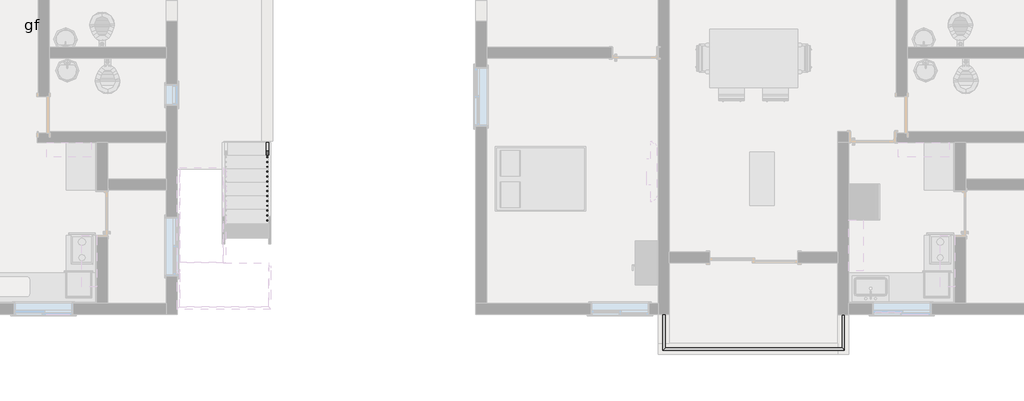
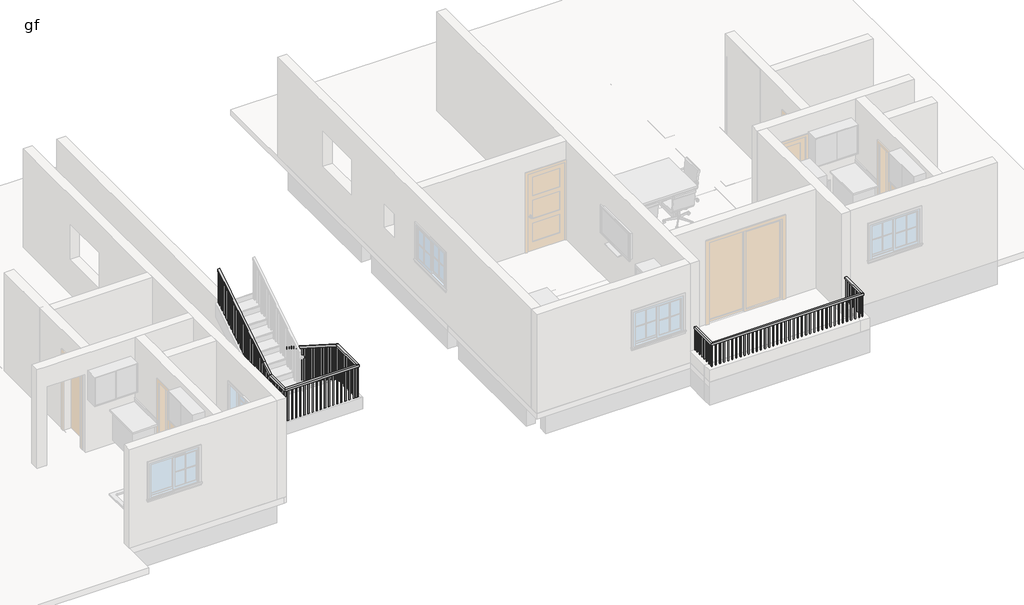
# One storey, part 5 of 8: 2 railings.
"""IFC4 building model written with IfcOpenShell, lengths in millimetres."""

from ifc_helpers import new_model, si_unit, frame, origin, place, context, project, spatial, polyline, outline, extrude, faceted_brep, element, save

model = new_model("IFC4")

# Units and contexts
model_context = context("Model", 3, world=origin())
ifc_project = project(units=[si_unit("LENGTHUNIT", "METRE", prefix="MILLI")], contexts=[model_context])

# Site, building, storey
site = spatial("IfcSite", under=ifc_project)
building = spatial("IfcBuilding", under=site)
storey = spatial("IfcBuildingStorey", under=building, Name="gf", Elevation=609.6)

# Railings
placement = place(None, origin())
element("IfcRailing", 1, ObjectType="Handrail - Rectangular", at=placement, inside=storey, context=model_context, shape_type="SolidModel", body=[
    faceted_brep([(5523.6761273, -4611.6564015, 1524.0), (5523.6761273, -4611.6564015, 1473.2), (5472.8761273, -4611.6564015, 1473.2), (5472.8761273, -4611.6564015, 1524.0), (5523.6761273, -5303.8064015, 1524.0), (5523.6761273, -5303.8064015, 1473.2), (5472.8761273, -5354.6064015, 1473.2), (5472.8761273, -5354.6064015, 1524.0), (9206.6761273, -5303.8064015, 1524.0), (9206.6761273, -5303.8064015, 1473.2), (9257.4761273, -5354.6064015, 1473.2), (9257.4761273, -5354.6064015, 1524.0), (9206.6761273, -4618.0064015, 1524.0), (9257.4761273, -4618.0064015, 1524.0), (9257.4761273, -4618.0064015, 1473.2), (9206.6761273, -4618.0064015, 1473.2)], [[[0, 1, 2, 3]], [[1, 0, 4, 5]], [[2, 1, 5, 6]], [[3, 2, 6, 7]], [[0, 3, 7, 4]], [[5, 4, 8, 9]], [[6, 5, 9, 10]], [[7, 6, 10, 11]], [[4, 7, 11, 8]], [[12, 13, 14, 15]], [[9, 8, 12, 15]], [[10, 9, 15, 14]], [[11, 10, 14, 13]], [[8, 11, 13, 12]]]),
    extrude(outline(polyline([(9241.6011273, -4729.1314015), (9222.5511273, -4729.1314015), (9222.5511273, -4710.0814015), (9241.6011273, -4710.0814015), (9241.6011273, -4729.1314015)])), frame((0.0, 0.0, 609.6), z_axis=(0.0, 0.0, 1.0), x_axis=(1.0, 0.0, 0.0)), (0.0, 0.0, 1.0), 863.6),
    extrude(outline(polyline([(9241.6011273, -4830.7314015), (9222.5511273, -4830.7314015), (9222.5511273, -4811.6814015), (9241.6011273, -4811.6814015), (9241.6011273, -4830.7314015)])), frame((0.0, 0.0, 609.6), z_axis=(0.0, 0.0, 1.0), x_axis=(1.0, 0.0, 0.0)), (0.0, 0.0, 1.0), 863.6),
    extrude(outline(polyline([(9241.6011273, -4932.3314015), (9222.5511273, -4932.3314015), (9222.5511273, -4913.2814015), (9241.6011273, -4913.2814015), (9241.6011273, -4932.3314015)])), frame((0.0, 0.0, 609.6), z_axis=(0.0, 0.0, 1.0), x_axis=(1.0, 0.0, 0.0)), (0.0, 0.0, 1.0), 863.6),
    extrude(outline(polyline([(9241.6011273, -5033.9314015), (9222.5511273, -5033.9314015), (9222.5511273, -5014.8814015), (9241.6011273, -5014.8814015), (9241.6011273, -5033.9314015)])), frame((0.0, 0.0, 609.6), z_axis=(0.0, 0.0, 1.0), x_axis=(1.0, 0.0, 0.0)), (0.0, 0.0, 1.0), 863.6),
    extrude(outline(polyline([(9241.6011273, -5135.5314015), (9222.5511273, -5135.5314015), (9222.5511273, -5116.4814015), (9241.6011273, -5116.4814015), (9241.6011273, -5135.5314015)])), frame((0.0, 0.0, 609.6), z_axis=(0.0, 0.0, 1.0), x_axis=(1.0, 0.0, 0.0)), (0.0, 0.0, 1.0), 863.6),
    extrude(outline(polyline([(9241.6011273, -5237.1314015), (9222.5511273, -5237.1314015), (9222.5511273, -5218.0814015), (9241.6011273, -5218.0814015), (9241.6011273, -5237.1314015)])), frame((0.0, 0.0, 609.6), z_axis=(0.0, 0.0, 1.0), x_axis=(1.0, 0.0, 0.0)), (0.0, 0.0, 1.0), 863.6),
    extrude(outline(polyline([(9146.3511273, -5338.7314015), (9146.3511273, -5319.6814015), (9165.4011273, -5319.6814015), (9165.4011273, -5338.7314015), (9146.3511273, -5338.7314015)])), frame((0.0, 0.0, 609.6), z_axis=(0.0, 0.0, 1.0), x_axis=(1.0, 0.0, 0.0)), (0.0, 0.0, 1.0), 863.6),
    extrude(outline(polyline([(9044.7511273, -5338.7314015), (9044.7511273, -5319.6814015), (9063.8011273, -5319.6814015), (9063.8011273, -5338.7314015), (9044.7511273, -5338.7314015)])), frame((0.0, 0.0, 609.6), z_axis=(0.0, 0.0, 1.0), x_axis=(1.0, 0.0, 0.0)), (0.0, 0.0, 1.0), 863.6),
    extrude(outline(polyline([(8943.1511273, -5338.7314015), (8943.1511273, -5319.6814015), (8962.2011273, -5319.6814015), (8962.2011273, -5338.7314015), (8943.1511273, -5338.7314015)])), frame((0.0, 0.0, 609.6), z_axis=(0.0, 0.0, 1.0), x_axis=(1.0, 0.0, 0.0)), (0.0, 0.0, 1.0), 863.6),
    extrude(outline(polyline([(8841.5511273, -5338.7314015), (8841.5511273, -5319.6814015), (8860.6011273, -5319.6814015), (8860.6011273, -5338.7314015), (8841.5511273, -5338.7314015)])), frame((0.0, 0.0, 609.6), z_axis=(0.0, 0.0, 1.0), x_axis=(1.0, 0.0, 0.0)), (0.0, 0.0, 1.0), 863.6),
    extrude(outline(polyline([(8739.9511273, -5338.7314015), (8739.9511273, -5319.6814015), (8759.0011273, -5319.6814015), (8759.0011273, -5338.7314015), (8739.9511273, -5338.7314015)])), frame((0.0, 0.0, 609.6), z_axis=(0.0, 0.0, 1.0), x_axis=(1.0, 0.0, 0.0)), (0.0, 0.0, 1.0), 863.6),
    extrude(outline(polyline([(8638.3511273, -5338.7314015), (8638.3511273, -5319.6814015), (8657.4011273, -5319.6814015), (8657.4011273, -5338.7314015), (8638.3511273, -5338.7314015)])), frame((0.0, 0.0, 609.6), z_axis=(0.0, 0.0, 1.0), x_axis=(1.0, 0.0, 0.0)), (0.0, 0.0, 1.0), 863.6),
    extrude(outline(polyline([(8536.7511273, -5338.7314015), (8536.7511273, -5319.6814015), (8555.8011273, -5319.6814015), (8555.8011273, -5338.7314015), (8536.7511273, -5338.7314015)])), frame((0.0, 0.0, 609.6), z_axis=(0.0, 0.0, 1.0), x_axis=(1.0, 0.0, 0.0)), (0.0, 0.0, 1.0), 863.6),
    extrude(outline(polyline([(8435.1511273, -5338.7314015), (8435.1511273, -5319.6814015), (8454.2011273, -5319.6814015), (8454.2011273, -5338.7314015), (8435.1511273, -5338.7314015)])), frame((0.0, 0.0, 609.6), z_axis=(0.0, 0.0, 1.0), x_axis=(1.0, 0.0, 0.0)), (0.0, 0.0, 1.0), 863.6),
    extrude(outline(polyline([(8333.5511273, -5338.7314015), (8333.5511273, -5319.6814015), (8352.6011273, -5319.6814015), (8352.6011273, -5338.7314015), (8333.5511273, -5338.7314015)])), frame((0.0, 0.0, 609.6), z_axis=(0.0, 0.0, 1.0), x_axis=(1.0, 0.0, 0.0)), (0.0, 0.0, 1.0), 863.6),
    extrude(outline(polyline([(8231.9511273, -5338.7314015), (8231.9511273, -5319.6814015), (8251.0011273, -5319.6814015), (8251.0011273, -5338.7314015), (8231.9511273, -5338.7314015)])), frame((0.0, 0.0, 609.6), z_axis=(0.0, 0.0, 1.0), x_axis=(1.0, 0.0, 0.0)), (0.0, 0.0, 1.0), 863.6),
    extrude(outline(polyline([(8130.3511273, -5338.7314015), (8130.3511273, -5319.6814015), (8149.4011273, -5319.6814015), (8149.4011273, -5338.7314015), (8130.3511273, -5338.7314015)])), frame((0.0, 0.0, 609.6), z_axis=(0.0, 0.0, 1.0), x_axis=(1.0, 0.0, 0.0)), (0.0, 0.0, 1.0), 863.6),
    extrude(outline(polyline([(8028.7511273, -5338.7314015), (8028.7511273, -5319.6814015), (8047.8011273, -5319.6814015), (8047.8011273, -5338.7314015), (8028.7511273, -5338.7314015)])), frame((0.0, 0.0, 609.6), z_axis=(0.0, 0.0, 1.0), x_axis=(1.0, 0.0, 0.0)), (0.0, 0.0, 1.0), 863.6),
    extrude(outline(polyline([(7927.1511273, -5338.7314015), (7927.1511273, -5319.6814015), (7946.2011273, -5319.6814015), (7946.2011273, -5338.7314015), (7927.1511273, -5338.7314015)])), frame((0.0, 0.0, 609.6), z_axis=(0.0, 0.0, 1.0), x_axis=(1.0, 0.0, 0.0)), (0.0, 0.0, 1.0), 863.6),
    extrude(outline(polyline([(7825.5511273, -5338.7314015), (7825.5511273, -5319.6814015), (7844.6011273, -5319.6814015), (7844.6011273, -5338.7314015), (7825.5511273, -5338.7314015)])), frame((0.0, 0.0, 609.6), z_axis=(0.0, 0.0, 1.0), x_axis=(1.0, 0.0, 0.0)), (0.0, 0.0, 1.0), 863.6),
    extrude(outline(polyline([(7723.9511273, -5338.7314015), (7723.9511273, -5319.6814015), (7743.0011273, -5319.6814015), (7743.0011273, -5338.7314015), (7723.9511273, -5338.7314015)])), frame((0.0, 0.0, 609.6), z_axis=(0.0, 0.0, 1.0), x_axis=(1.0, 0.0, 0.0)), (0.0, 0.0, 1.0), 863.6),
    extrude(outline(polyline([(7622.3511273, -5338.7314015), (7622.3511273, -5319.6814015), (7641.4011273, -5319.6814015), (7641.4011273, -5338.7314015), (7622.3511273, -5338.7314015)])), frame((0.0, 0.0, 609.6), z_axis=(0.0, 0.0, 1.0), x_axis=(1.0, 0.0, 0.0)), (0.0, 0.0, 1.0), 863.6),
    extrude(outline(polyline([(7520.7511273, -5338.7314015), (7520.7511273, -5319.6814015), (7539.8011273, -5319.6814015), (7539.8011273, -5338.7314015), (7520.7511273, -5338.7314015)])), frame((0.0, 0.0, 609.6), z_axis=(0.0, 0.0, 1.0), x_axis=(1.0, 0.0, 0.0)), (0.0, 0.0, 1.0), 863.6),
    extrude(outline(polyline([(7419.1511273, -5338.7314015), (7419.1511273, -5319.6814015), (7438.2011273, -5319.6814015), (7438.2011273, -5338.7314015), (7419.1511273, -5338.7314015)])), frame((0.0, 0.0, 609.6), z_axis=(0.0, 0.0, 1.0), x_axis=(1.0, 0.0, 0.0)), (0.0, 0.0, 1.0), 863.6),
    extrude(outline(polyline([(7317.5511273, -5338.7314015), (7317.5511273, -5319.6814015), (7336.6011273, -5319.6814015), (7336.6011273, -5338.7314015), (7317.5511273, -5338.7314015)])), frame((0.0, 0.0, 609.6), z_axis=(0.0, 0.0, 1.0), x_axis=(1.0, 0.0, 0.0)), (0.0, 0.0, 1.0), 863.6),
    extrude(outline(polyline([(7215.9511273, -5338.7314015), (7215.9511273, -5319.6814015), (7235.0011273, -5319.6814015), (7235.0011273, -5338.7314015), (7215.9511273, -5338.7314015)])), frame((0.0, 0.0, 609.6), z_axis=(0.0, 0.0, 1.0), x_axis=(1.0, 0.0, 0.0)), (0.0, 0.0, 1.0), 863.6),
    extrude(outline(polyline([(7114.3511273, -5338.7314015), (7114.3511273, -5319.6814015), (7133.4011273, -5319.6814015), (7133.4011273, -5338.7314015), (7114.3511273, -5338.7314015)])), frame((0.0, 0.0, 609.6), z_axis=(0.0, 0.0, 1.0), x_axis=(1.0, 0.0, 0.0)), (0.0, 0.0, 1.0), 863.6),
    extrude(outline(polyline([(7012.7511273, -5338.7314015), (7012.7511273, -5319.6814015), (7031.8011273, -5319.6814015), (7031.8011273, -5338.7314015), (7012.7511273, -5338.7314015)])), frame((0.0, 0.0, 609.6), z_axis=(0.0, 0.0, 1.0), x_axis=(1.0, 0.0, 0.0)), (0.0, 0.0, 1.0), 863.6),
    extrude(outline(polyline([(6911.1511273, -5338.7314015), (6911.1511273, -5319.6814015), (6930.2011273, -5319.6814015), (6930.2011273, -5338.7314015), (6911.1511273, -5338.7314015)])), frame((0.0, 0.0, 609.6), z_axis=(0.0, 0.0, 1.0), x_axis=(1.0, 0.0, 0.0)), (0.0, 0.0, 1.0), 863.6),
    extrude(outline(polyline([(6809.5511273, -5338.7314015), (6809.5511273, -5319.6814015), (6828.6011273, -5319.6814015), (6828.6011273, -5338.7314015), (6809.5511273, -5338.7314015)])), frame((0.0, 0.0, 609.6), z_axis=(0.0, 0.0, 1.0), x_axis=(1.0, 0.0, 0.0)), (0.0, 0.0, 1.0), 863.6),
    extrude(outline(polyline([(6707.9511273, -5338.7314015), (6707.9511273, -5319.6814015), (6727.0011273, -5319.6814015), (6727.0011273, -5338.7314015), (6707.9511273, -5338.7314015)])), frame((0.0, 0.0, 609.6), z_axis=(0.0, 0.0, 1.0), x_axis=(1.0, 0.0, 0.0)), (0.0, 0.0, 1.0), 863.6),
    extrude(outline(polyline([(6606.3511273, -5338.7314015), (6606.3511273, -5319.6814015), (6625.4011273, -5319.6814015), (6625.4011273, -5338.7314015), (6606.3511273, -5338.7314015)])), frame((0.0, 0.0, 609.6), z_axis=(0.0, 0.0, 1.0), x_axis=(1.0, 0.0, 0.0)), (0.0, 0.0, 1.0), 863.6),
    extrude(outline(polyline([(6504.7511273, -5338.7314015), (6504.7511273, -5319.6814015), (6523.8011273, -5319.6814015), (6523.8011273, -5338.7314015), (6504.7511273, -5338.7314015)])), frame((0.0, 0.0, 609.6), z_axis=(0.0, 0.0, 1.0), x_axis=(1.0, 0.0, 0.0)), (0.0, 0.0, 1.0), 863.6),
    extrude(outline(polyline([(6403.1511273, -5338.7314015), (6403.1511273, -5319.6814015), (6422.2011273, -5319.6814015), (6422.2011273, -5338.7314015), (6403.1511273, -5338.7314015)])), frame((0.0, 0.0, 609.6), z_axis=(0.0, 0.0, 1.0), x_axis=(1.0, 0.0, 0.0)), (0.0, 0.0, 1.0), 863.6),
    extrude(outline(polyline([(6301.5511273, -5338.7314015), (6301.5511273, -5319.6814015), (6320.6011273, -5319.6814015), (6320.6011273, -5338.7314015), (6301.5511273, -5338.7314015)])), frame((0.0, 0.0, 609.6), z_axis=(0.0, 0.0, 1.0), x_axis=(1.0, 0.0, 0.0)), (0.0, 0.0, 1.0), 863.6),
    extrude(outline(polyline([(6199.9511273, -5338.7314015), (6199.9511273, -5319.6814015), (6219.0011273, -5319.6814015), (6219.0011273, -5338.7314015), (6199.9511273, -5338.7314015)])), frame((0.0, 0.0, 609.6), z_axis=(0.0, 0.0, 1.0), x_axis=(1.0, 0.0, 0.0)), (0.0, 0.0, 1.0), 863.6),
    extrude(outline(polyline([(6098.3511273, -5338.7314015), (6098.3511273, -5319.6814015), (6117.4011273, -5319.6814015), (6117.4011273, -5338.7314015), (6098.3511273, -5338.7314015)])), frame((0.0, 0.0, 609.6), z_axis=(0.0, 0.0, 1.0), x_axis=(1.0, 0.0, 0.0)), (0.0, 0.0, 1.0), 863.6),
    extrude(outline(polyline([(5996.7511273, -5338.7314015), (5996.7511273, -5319.6814015), (6015.8011273, -5319.6814015), (6015.8011273, -5338.7314015), (5996.7511273, -5338.7314015)])), frame((0.0, 0.0, 609.6), z_axis=(0.0, 0.0, 1.0), x_axis=(1.0, 0.0, 0.0)), (0.0, 0.0, 1.0), 863.6),
    extrude(outline(polyline([(5895.1511273, -5338.7314015), (5895.1511273, -5319.6814015), (5914.2011273, -5319.6814015), (5914.2011273, -5338.7314015), (5895.1511273, -5338.7314015)])), frame((0.0, 0.0, 609.6), z_axis=(0.0, 0.0, 1.0), x_axis=(1.0, 0.0, 0.0)), (0.0, 0.0, 1.0), 863.6),
    extrude(outline(polyline([(5793.5511273, -5338.7314015), (5793.5511273, -5319.6814015), (5812.6011273, -5319.6814015), (5812.6011273, -5338.7314015), (5793.5511273, -5338.7314015)])), frame((0.0, 0.0, 609.6), z_axis=(0.0, 0.0, 1.0), x_axis=(1.0, 0.0, 0.0)), (0.0, 0.0, 1.0), 863.6),
    extrude(outline(polyline([(5691.9511273, -5338.7314015), (5691.9511273, -5319.6814015), (5711.0011273, -5319.6814015), (5711.0011273, -5338.7314015), (5691.9511273, -5338.7314015)])), frame((0.0, 0.0, 609.6), z_axis=(0.0, 0.0, 1.0), x_axis=(1.0, 0.0, 0.0)), (0.0, 0.0, 1.0), 863.6),
    extrude(outline(polyline([(5590.3511273, -5338.7314015), (5590.3511273, -5319.6814015), (5609.4011273, -5319.6814015), (5609.4011273, -5338.7314015), (5590.3511273, -5338.7314015)])), frame((0.0, 0.0, 609.6), z_axis=(0.0, 0.0, 1.0), x_axis=(1.0, 0.0, 0.0)), (0.0, 0.0, 1.0), 863.6),
    extrude(outline(polyline([(5488.7511273, -5313.3314015), (5507.8011273, -5313.3314015), (5507.8011273, -5332.3814015), (5488.7511273, -5332.3814015), (5488.7511273, -5313.3314015)])), frame((0.0, 0.0, 609.6), z_axis=(0.0, 0.0, 1.0), x_axis=(1.0, 0.0, 0.0)), (0.0, 0.0, 1.0), 863.6),
    extrude(outline(polyline([(5488.7511273, -5211.7314015), (5507.8011273, -5211.7314015), (5507.8011273, -5230.7814015), (5488.7511273, -5230.7814015), (5488.7511273, -5211.7314015)])), frame((0.0, 0.0, 609.6), z_axis=(0.0, 0.0, 1.0), x_axis=(1.0, 0.0, 0.0)), (0.0, 0.0, 1.0), 863.6),
    extrude(outline(polyline([(5488.7511273, -5110.1314015), (5507.8011273, -5110.1314015), (5507.8011273, -5129.1814015), (5488.7511273, -5129.1814015), (5488.7511273, -5110.1314015)])), frame((0.0, 0.0, 609.6), z_axis=(0.0, 0.0, 1.0), x_axis=(1.0, 0.0, 0.0)), (0.0, 0.0, 1.0), 863.6),
    extrude(outline(polyline([(5488.7511273, -5008.5314015), (5507.8011273, -5008.5314015), (5507.8011273, -5027.5814015), (5488.7511273, -5027.5814015), (5488.7511273, -5008.5314015)])), frame((0.0, 0.0, 609.6), z_axis=(0.0, 0.0, 1.0), x_axis=(1.0, 0.0, 0.0)), (0.0, 0.0, 1.0), 863.6),
    extrude(outline(polyline([(5488.7511273, -4906.9314015), (5507.8011273, -4906.9314015), (5507.8011273, -4925.9814015), (5488.7511273, -4925.9814015), (5488.7511273, -4906.9314015)])), frame((0.0, 0.0, 609.6), z_axis=(0.0, 0.0, 1.0), x_axis=(1.0, 0.0, 0.0)), (0.0, 0.0, 1.0), 863.6),
    extrude(outline(polyline([(5488.7511273, -4805.3314015), (5507.8011273, -4805.3314015), (5507.8011273, -4824.3814015), (5488.7511273, -4824.3814015), (5488.7511273, -4805.3314015)])), frame((0.0, 0.0, 609.6), z_axis=(0.0, 0.0, 1.0), x_axis=(1.0, 0.0, 0.0)), (0.0, 0.0, 1.0), 863.6),
    extrude(outline(polyline([(5488.7511273, -4703.7314015), (5507.8011273, -4703.7314015), (5507.8011273, -4722.7814015), (5488.7511273, -4722.7814015), (5488.7511273, -4703.7314015)])), frame((0.0, 0.0, 609.6), z_axis=(0.0, 0.0, 1.0), x_axis=(1.0, 0.0, 0.0)), (0.0, 0.0, 1.0), 863.6),
    extrude(outline(polyline([(9222.5511273, -5338.7314015), (9222.5511273, -5319.6814015), (9241.6011273, -5319.6814015), (9241.6011273, -5338.7314015), (9222.5511273, -5338.7314015)])), frame((0.0, 0.0, 609.6), z_axis=(0.0, 0.0, 1.0), x_axis=(1.0, 0.0, 0.0)), (0.0, 0.0, 1.0), 863.6),
    extrude(outline(polyline([(5488.7511273, -5319.6814015), (5507.8011273, -5319.6814015), (5507.8011273, -5338.7314015), (5488.7511273, -5338.7314015), (5488.7511273, -5319.6814015)])), frame((0.0, 0.0, 609.6), z_axis=(0.0, 0.0, 1.0), x_axis=(1.0, 0.0, 0.0)), (0.0, 0.0, 1.0), 863.6),
    extrude(outline(polyline([(9241.6011273, -4637.0564015), (9222.5511273, -4637.0564015), (9222.5511273, -4618.0064015), (9241.6011273, -4618.0064015), (9241.6011273, -4637.0564015)])), frame((0.0, 0.0, 609.6), z_axis=(0.0, 0.0, 1.0), x_axis=(1.0, 0.0, 0.0)), (0.0, 0.0, 1.0), 863.6),
    extrude(outline(polyline([(5488.7511273, -4611.6564015), (5507.8011273, -4611.6564015), (5507.8011273, -4630.7064015), (5488.7511273, -4630.7064015), (5488.7511273, -4611.6564015)])), frame((0.0, 0.0, 609.6), z_axis=(0.0, 0.0, 1.0), x_axis=(1.0, 0.0, 0.0)), (0.0, 0.0, 1.0), 863.6),
])
element("IfcRailing", 2, ObjectType="Handrail - Rectangular", at=placement, inside=storey, context=model_context, shape_type="SolidModel", body=[
    faceted_brep([(-2736.9993763, -1023.9064015, 1701.8), (-2736.9993763, -1023.9064015, 1641.586276), (-2787.7993763, -1023.9064015, 1641.586276), (-2787.7993763, -1023.9064015, 1701.8), (-2736.9993763, -3538.5064015, 3302.0), (-2736.9993763, -3553.2993964, 3251.2), (-2787.7993763, -3553.2993964, 3251.2), (-2787.7993763, -3538.5064015, 3302.0), (-2736.9993763, -4452.9064015, 3302.0), (-2736.9993763, -4452.9064015, 3251.2), (-2787.7993763, -4402.1064015, 3251.2), (-2787.7993763, -4402.1064015, 3302.0), (-4591.1993763, -4452.9064015, 3302.0), (-4591.1993763, -4452.9064015, 3251.2), (-4540.3993763, -4402.1064015, 3251.2), (-4540.3993763, -4402.1064015, 3302.0), (-4591.1993763, -3817.9064015, 3302.0), (-4591.1993763, -3803.1134066, 3251.2), (-4540.3993763, -3803.1134066, 3251.2), (-4540.3993763, -3817.9064015, 3302.0), (-4591.1993763, -3538.5064015, 3479.8), (-4591.1993763, -3511.2331265, 3436.9419964), (-4540.3993763, -3511.2331265, 3436.9419964), (-4540.3993763, -3538.5064015, 3479.8), (-4591.1993763, -1582.7064015, 4724.4), (-4540.3993763, -1582.7064015, 4724.4), (-4540.3993763, -1582.7064015, 4664.186276), (-4591.1993763, -1582.7064015, 4664.186276)], [[[0, 1, 2, 3]], [[1, 0, 4, 5]], [[2, 1, 5, 6]], [[3, 2, 6, 7]], [[0, 3, 7, 4]], [[5, 4, 8, 9]], [[6, 5, 9, 10]], [[7, 6, 10, 11]], [[4, 7, 11, 8]], [[9, 8, 12, 13]], [[10, 9, 13, 14]], [[11, 10, 14, 15]], [[8, 11, 15, 12]], [[13, 12, 16, 17]], [[14, 13, 17, 18]], [[15, 14, 18, 19]], [[12, 15, 19, 16]], [[17, 16, 20, 21]], [[18, 17, 21, 22]], [[19, 18, 22, 23]], [[16, 19, 23, 20]], [[24, 25, 26, 27]], [[21, 20, 24, 27]], [[22, 21, 27, 26]], [[23, 22, 26, 25]], [[20, 23, 25, 24]]]),
    extrude(outline(polyline([(-1598.5814015, 4654.0840032), (-1598.5814015, 3632.2), (-1617.6314015, 3632.2), (-1617.6314015, 4641.961276), (-1598.5814015, 4654.0840032)])), frame((-4575.3243763, 0.0, 0.0), z_axis=(1.0, 0.0, 0.0), x_axis=(0.0, 1.0, 0.0)), (0.0, 0.0, 1.0), 19.05),
    extrude(outline(polyline([(-1700.1814015, 4589.4294578), (-1700.1814015, 3632.2), (-1719.2314015, 3632.2), (-1719.2314015, 4577.3067305), (-1700.1814015, 4589.4294578)])), frame((-4575.3243763, 0.0, 0.0), z_axis=(1.0, 0.0, 0.0), x_axis=(0.0, 1.0, 0.0)), (0.0, 0.0, 1.0), 19.05),
    extrude(outline(polyline([(-1801.7814015, 4524.7749123), (-1801.7814015, 3632.2), (-1820.8314015, 3632.2), (-1820.8314015, 4512.6521851), (-1801.7814015, 4524.7749123)])), frame((-4575.3243763, 0.0, 0.0), z_axis=(1.0, 0.0, 0.0), x_axis=(0.0, 1.0, 0.0)), (0.0, 0.0, 1.0), 19.05),
    extrude(outline(polyline([(-1903.3814015, 4460.1203669), (-1903.3814015, 3454.4), (-1922.4314015, 3454.4), (-1922.4314015, 4447.9976396), (-1903.3814015, 4460.1203669)])), frame((-4575.3243763, 0.0, 0.0), z_axis=(1.0, 0.0, 0.0), x_axis=(0.0, 1.0, 0.0)), (0.0, 0.0, 1.0), 19.05),
    extrude(outline(polyline([(-2004.9814015, 4395.4658214), (-2004.9814015, 3454.4), (-2024.0314015, 3454.4), (-2024.0314015, 4383.3430941), (-2004.9814015, 4395.4658214)])), frame((-4575.3243763, 0.0, 0.0), z_axis=(1.0, 0.0, 0.0), x_axis=(0.0, 1.0, 0.0)), (0.0, 0.0, 1.0), 19.05),
    extrude(outline(polyline([(-2106.5814015, 4330.811276), (-2106.5814015, 3454.4), (-2125.6314015, 3454.4), (-2125.6314015, 4318.6885487), (-2106.5814015, 4330.811276)])), frame((-4575.3243763, 0.0, 0.0), z_axis=(1.0, 0.0, 0.0), x_axis=(0.0, 1.0, 0.0)), (0.0, 0.0, 1.0), 19.05),
    extrude(outline(polyline([(-2208.1814015, 4266.1567305), (-2208.1814015, 3276.6), (-2227.2314015, 3276.6), (-2227.2314015, 4254.0340032), (-2208.1814015, 4266.1567305)])), frame((-4575.3243763, 0.0, 0.0), z_axis=(1.0, 0.0, 0.0), x_axis=(0.0, 1.0, 0.0)), (0.0, 0.0, 1.0), 19.05),
    extrude(outline(polyline([(-2309.7814015, 4201.5021851), (-2309.7814015, 3276.6), (-2328.8314015, 3276.6), (-2328.8314015, 4189.3794578), (-2309.7814015, 4201.5021851)])), frame((-4575.3243763, 0.0, 0.0), z_axis=(1.0, 0.0, 0.0), x_axis=(0.0, 1.0, 0.0)), (0.0, 0.0, 1.0), 19.05),
    extrude(outline(polyline([(-2411.3814015, 4136.8476396), (-2411.3814015, 3276.6), (-2430.4314015, 3276.6), (-2430.4314015, 4124.7249123), (-2411.3814015, 4136.8476396)])), frame((-4575.3243763, 0.0, 0.0), z_axis=(1.0, 0.0, 0.0), x_axis=(0.0, 1.0, 0.0)), (0.0, 0.0, 1.0), 19.05),
    extrude(outline(polyline([(-2512.9814015, 4072.1930941), (-2512.9814015, 3098.8), (-2532.0314015, 3098.8), (-2532.0314015, 4060.0703669), (-2512.9814015, 4072.1930941)])), frame((-4575.3243763, 0.0, 0.0), z_axis=(1.0, 0.0, 0.0), x_axis=(0.0, 1.0, 0.0)), (0.0, 0.0, 1.0), 19.05),
    extrude(outline(polyline([(-2614.5814015, 4007.5385487), (-2614.5814015, 3098.8), (-2633.6314015, 3098.8), (-2633.6314015, 3995.4158214), (-2614.5814015, 4007.5385487)])), frame((-4575.3243763, 0.0, 0.0), z_axis=(1.0, 0.0, 0.0), x_axis=(0.0, 1.0, 0.0)), (0.0, 0.0, 1.0), 19.05),
    extrude(outline(polyline([(-2716.1814015, 3942.8840032), (-2716.1814015, 2921.0), (-2735.2314015, 2921.0), (-2735.2314015, 3930.761276), (-2716.1814015, 3942.8840032)])), frame((-4575.3243763, 0.0, 0.0), z_axis=(1.0, 0.0, 0.0), x_axis=(0.0, 1.0, 0.0)), (0.0, 0.0, 1.0), 19.05),
    extrude(outline(polyline([(-2817.7814015, 3878.2294578), (-2817.7814015, 2921.0), (-2836.8314015, 2921.0), (-2836.8314015, 3866.1067305), (-2817.7814015, 3878.2294578)])), frame((-4575.3243763, 0.0, 0.0), z_axis=(1.0, 0.0, 0.0), x_axis=(0.0, 1.0, 0.0)), (0.0, 0.0, 1.0), 19.05),
    extrude(outline(polyline([(-2919.3814015, 3813.5749123), (-2919.3814015, 2921.0), (-2938.4314015, 2921.0), (-2938.4314015, 3801.4521851), (-2919.3814015, 3813.5749123)])), frame((-4575.3243763, 0.0, 0.0), z_axis=(1.0, 0.0, 0.0), x_axis=(0.0, 1.0, 0.0)), (0.0, 0.0, 1.0), 19.05),
    extrude(outline(polyline([(-3020.9814015, 3748.9203669), (-3020.9814015, 2743.2), (-3040.0314015, 2743.2), (-3040.0314015, 3736.7976396), (-3020.9814015, 3748.9203669)])), frame((-4575.3243763, 0.0, 0.0), z_axis=(1.0, 0.0, 0.0), x_axis=(0.0, 1.0, 0.0)), (0.0, 0.0, 1.0), 19.05),
    extrude(outline(polyline([(-3122.5814015, 3684.2658214), (-3122.5814015, 2743.2), (-3141.6314015, 2743.2), (-3141.6314015, 3672.1430941), (-3122.5814015, 3684.2658214)])), frame((-4575.3243763, 0.0, 0.0), z_axis=(1.0, 0.0, 0.0), x_axis=(0.0, 1.0, 0.0)), (0.0, 0.0, 1.0), 19.05),
    extrude(outline(polyline([(-3224.1814015, 3619.611276), (-3224.1814015, 2743.2), (-3243.2314015, 2743.2), (-3243.2314015, 3607.4885487), (-3224.1814015, 3619.611276)])), frame((-4575.3243763, 0.0, 0.0), z_axis=(1.0, 0.0, 0.0), x_axis=(0.0, 1.0, 0.0)), (0.0, 0.0, 1.0), 19.05),
    extrude(outline(polyline([(-3325.7814015, 3554.9567305), (-3325.7814015, 2565.4), (-3344.8314015, 2565.4), (-3344.8314015, 3542.8340032), (-3325.7814015, 3554.9567305)])), frame((-4575.3243763, 0.0, 0.0), z_axis=(1.0, 0.0, 0.0), x_axis=(0.0, 1.0, 0.0)), (0.0, 0.0, 1.0), 19.05),
    extrude(outline(polyline([(-3427.3814015, 3490.3021851), (-3427.3814015, 2565.4), (-3446.4314015, 2565.4), (-3446.4314015, 3478.1794578), (-3427.3814015, 3490.3021851)])), frame((-4575.3243763, 0.0, 0.0), z_axis=(1.0, 0.0, 0.0), x_axis=(0.0, 1.0, 0.0)), (0.0, 0.0, 1.0), 19.05),
    extrude(outline(polyline([(-3605.1814015, 3377.1567305), (-3605.1814015, 2387.6), (-3624.2314015, 2387.6), (-3624.2314015, 3365.0340032), (-3605.1814015, 3377.1567305)])), frame((-4575.3243763, 0.0, 0.0), z_axis=(1.0, 0.0, 0.0), x_axis=(0.0, 1.0, 0.0)), (0.0, 0.0, 1.0), 19.05),
    extrude(outline(polyline([(-3706.7814015, 3312.5021851), (-3706.7814015, 2387.6), (-3725.8314015, 2387.6), (-3725.8314015, 3300.3794578), (-3706.7814015, 3312.5021851)])), frame((-4575.3243763, 0.0, 0.0), z_axis=(1.0, 0.0, 0.0), x_axis=(0.0, 1.0, 0.0)), (0.0, 0.0, 1.0), 19.05),
    extrude(outline(polyline([(-4575.3243763, -3827.4314015), (-4575.3243763, -3808.3814015), (-4556.2743763, -3808.3814015), (-4556.2743763, -3827.4314015), (-4575.3243763, -3827.4314015)])), frame((0.0, 0.0, 2387.6), z_axis=(0.0, 0.0, 1.0), x_axis=(1.0, 0.0, 0.0)), (0.0, 0.0, 1.0), 863.6),
    extrude(outline(polyline([(-4575.3243763, -3929.0314015), (-4575.3243763, -3909.9814015), (-4556.2743763, -3909.9814015), (-4556.2743763, -3929.0314015), (-4575.3243763, -3929.0314015)])), frame((0.0, 0.0, 2387.6), z_axis=(0.0, 0.0, 1.0), x_axis=(1.0, 0.0, 0.0)), (0.0, 0.0, 1.0), 863.6),
    extrude(outline(polyline([(-4575.3243763, -4030.6314015), (-4575.3243763, -4011.5814015), (-4556.2743763, -4011.5814015), (-4556.2743763, -4030.6314015), (-4575.3243763, -4030.6314015)])), frame((0.0, 0.0, 2387.6), z_axis=(0.0, 0.0, 1.0), x_axis=(1.0, 0.0, 0.0)), (0.0, 0.0, 1.0), 863.6),
    extrude(outline(polyline([(-4575.3243763, -4132.2314015), (-4575.3243763, -4113.1814015), (-4556.2743763, -4113.1814015), (-4556.2743763, -4132.2314015), (-4575.3243763, -4132.2314015)])), frame((0.0, 0.0, 2387.6), z_axis=(0.0, 0.0, 1.0), x_axis=(1.0, 0.0, 0.0)), (0.0, 0.0, 1.0), 863.6),
    extrude(outline(polyline([(-4575.3243763, -4233.8314015), (-4575.3243763, -4214.7814015), (-4556.2743763, -4214.7814015), (-4556.2743763, -4233.8314015), (-4575.3243763, -4233.8314015)])), frame((0.0, 0.0, 2387.6), z_axis=(0.0, 0.0, 1.0), x_axis=(1.0, 0.0, 0.0)), (0.0, 0.0, 1.0), 863.6),
    extrude(outline(polyline([(-4575.3243763, -4335.4314015), (-4575.3243763, -4316.3814015), (-4556.2743763, -4316.3814015), (-4556.2743763, -4335.4314015), (-4575.3243763, -4335.4314015)])), frame((0.0, 0.0, 2387.6), z_axis=(0.0, 0.0, 1.0), x_axis=(1.0, 0.0, 0.0)), (0.0, 0.0, 1.0), 863.6),
    extrude(outline(polyline([(-4480.0743763, -4437.0314015), (-4499.1243763, -4437.0314015), (-4499.1243763, -4417.9814015), (-4480.0743763, -4417.9814015), (-4480.0743763, -4437.0314015)])), frame((0.0, 0.0, 2387.6), z_axis=(0.0, 0.0, 1.0), x_axis=(1.0, 0.0, 0.0)), (0.0, 0.0, 1.0), 863.6),
    extrude(outline(polyline([(-4378.4743763, -4437.0314015), (-4397.5243763, -4437.0314015), (-4397.5243763, -4417.9814015), (-4378.4743763, -4417.9814015), (-4378.4743763, -4437.0314015)])), frame((0.0, 0.0, 2387.6), z_axis=(0.0, 0.0, 1.0), x_axis=(1.0, 0.0, 0.0)), (0.0, 0.0, 1.0), 863.6),
    extrude(outline(polyline([(-4276.8743763, -4437.0314015), (-4295.9243763, -4437.0314015), (-4295.9243763, -4417.9814015), (-4276.8743763, -4417.9814015), (-4276.8743763, -4437.0314015)])), frame((0.0, 0.0, 2387.6), z_axis=(0.0, 0.0, 1.0), x_axis=(1.0, 0.0, 0.0)), (0.0, 0.0, 1.0), 863.6),
    extrude(outline(polyline([(-4175.2743763, -4437.0314015), (-4194.3243763, -4437.0314015), (-4194.3243763, -4417.9814015), (-4175.2743763, -4417.9814015), (-4175.2743763, -4437.0314015)])), frame((0.0, 0.0, 2387.6), z_axis=(0.0, 0.0, 1.0), x_axis=(1.0, 0.0, 0.0)), (0.0, 0.0, 1.0), 863.6),
    extrude(outline(polyline([(-4073.6743763, -4437.0314015), (-4092.7243763, -4437.0314015), (-4092.7243763, -4417.9814015), (-4073.6743763, -4417.9814015), (-4073.6743763, -4437.0314015)])), frame((0.0, 0.0, 2387.6), z_axis=(0.0, 0.0, 1.0), x_axis=(1.0, 0.0, 0.0)), (0.0, 0.0, 1.0), 863.6),
    extrude(outline(polyline([(-3972.0743763, -4437.0314015), (-3991.1243763, -4437.0314015), (-3991.1243763, -4417.9814015), (-3972.0743763, -4417.9814015), (-3972.0743763, -4437.0314015)])), frame((0.0, 0.0, 2387.6), z_axis=(0.0, 0.0, 1.0), x_axis=(1.0, 0.0, 0.0)), (0.0, 0.0, 1.0), 863.6),
    extrude(outline(polyline([(-3870.4743763, -4437.0314015), (-3889.5243763, -4437.0314015), (-3889.5243763, -4417.9814015), (-3870.4743763, -4417.9814015), (-3870.4743763, -4437.0314015)])), frame((0.0, 0.0, 2387.6), z_axis=(0.0, 0.0, 1.0), x_axis=(1.0, 0.0, 0.0)), (0.0, 0.0, 1.0), 863.6),
    extrude(outline(polyline([(-3768.8743763, -4437.0314015), (-3787.9243763, -4437.0314015), (-3787.9243763, -4417.9814015), (-3768.8743763, -4417.9814015), (-3768.8743763, -4437.0314015)])), frame((0.0, 0.0, 2387.6), z_axis=(0.0, 0.0, 1.0), x_axis=(1.0, 0.0, 0.0)), (0.0, 0.0, 1.0), 863.6),
    extrude(outline(polyline([(-3667.2743763, -4437.0314015), (-3686.3243763, -4437.0314015), (-3686.3243763, -4417.9814015), (-3667.2743763, -4417.9814015), (-3667.2743763, -4437.0314015)])), frame((0.0, 0.0, 2387.6), z_axis=(0.0, 0.0, 1.0), x_axis=(1.0, 0.0, 0.0)), (0.0, 0.0, 1.0), 863.6),
    extrude(outline(polyline([(-3565.6743763, -4437.0314015), (-3584.7243763, -4437.0314015), (-3584.7243763, -4417.9814015), (-3565.6743763, -4417.9814015), (-3565.6743763, -4437.0314015)])), frame((0.0, 0.0, 2387.6), z_axis=(0.0, 0.0, 1.0), x_axis=(1.0, 0.0, 0.0)), (0.0, 0.0, 1.0), 863.6),
    extrude(outline(polyline([(-3464.0743763, -4437.0314015), (-3483.1243763, -4437.0314015), (-3483.1243763, -4417.9814015), (-3464.0743763, -4417.9814015), (-3464.0743763, -4437.0314015)])), frame((0.0, 0.0, 2387.6), z_axis=(0.0, 0.0, 1.0), x_axis=(1.0, 0.0, 0.0)), (0.0, 0.0, 1.0), 863.6),
    extrude(outline(polyline([(-3362.4743763, -4437.0314015), (-3381.5243763, -4437.0314015), (-3381.5243763, -4417.9814015), (-3362.4743763, -4417.9814015), (-3362.4743763, -4437.0314015)])), frame((0.0, 0.0, 2387.6), z_axis=(0.0, 0.0, 1.0), x_axis=(1.0, 0.0, 0.0)), (0.0, 0.0, 1.0), 863.6),
    extrude(outline(polyline([(-3260.8743763, -4437.0314015), (-3279.9243763, -4437.0314015), (-3279.9243763, -4417.9814015), (-3260.8743763, -4417.9814015), (-3260.8743763, -4437.0314015)])), frame((0.0, 0.0, 2387.6), z_axis=(0.0, 0.0, 1.0), x_axis=(1.0, 0.0, 0.0)), (0.0, 0.0, 1.0), 863.6),
    extrude(outline(polyline([(-3159.2743763, -4437.0314015), (-3178.3243763, -4437.0314015), (-3178.3243763, -4417.9814015), (-3159.2743763, -4417.9814015), (-3159.2743763, -4437.0314015)])), frame((0.0, 0.0, 2387.6), z_axis=(0.0, 0.0, 1.0), x_axis=(1.0, 0.0, 0.0)), (0.0, 0.0, 1.0), 863.6),
    extrude(outline(polyline([(-3057.6743763, -4437.0314015), (-3076.7243763, -4437.0314015), (-3076.7243763, -4417.9814015), (-3057.6743763, -4417.9814015), (-3057.6743763, -4437.0314015)])), frame((0.0, 0.0, 2387.6), z_axis=(0.0, 0.0, 1.0), x_axis=(1.0, 0.0, 0.0)), (0.0, 0.0, 1.0), 863.6),
    extrude(outline(polyline([(-2956.0743763, -4437.0314015), (-2975.1243763, -4437.0314015), (-2975.1243763, -4417.9814015), (-2956.0743763, -4417.9814015), (-2956.0743763, -4437.0314015)])), frame((0.0, 0.0, 2387.6), z_axis=(0.0, 0.0, 1.0), x_axis=(1.0, 0.0, 0.0)), (0.0, 0.0, 1.0), 863.6),
    extrude(outline(polyline([(-2854.4743763, -4437.0314015), (-2873.5243763, -4437.0314015), (-2873.5243763, -4417.9814015), (-2854.4743763, -4417.9814015), (-2854.4743763, -4437.0314015)])), frame((0.0, 0.0, 2387.6), z_axis=(0.0, 0.0, 1.0), x_axis=(1.0, 0.0, 0.0)), (0.0, 0.0, 1.0), 863.6),
    extrude(outline(polyline([(-2752.8743763, -4341.7814015), (-2752.8743763, -4360.8314015), (-2771.9243763, -4360.8314015), (-2771.9243763, -4341.7814015), (-2752.8743763, -4341.7814015)])), frame((0.0, 0.0, 2387.6), z_axis=(0.0, 0.0, 1.0), x_axis=(1.0, 0.0, 0.0)), (0.0, 0.0, 1.0), 863.6),
    extrude(outline(polyline([(-2752.8743763, -4240.1814015), (-2752.8743763, -4259.2314015), (-2771.9243763, -4259.2314015), (-2771.9243763, -4240.1814015), (-2752.8743763, -4240.1814015)])), frame((0.0, 0.0, 2387.6), z_axis=(0.0, 0.0, 1.0), x_axis=(1.0, 0.0, 0.0)), (0.0, 0.0, 1.0), 863.6),
    extrude(outline(polyline([(-2752.8743763, -4138.5814015), (-2752.8743763, -4157.6314015), (-2771.9243763, -4157.6314015), (-2771.9243763, -4138.5814015), (-2752.8743763, -4138.5814015)])), frame((0.0, 0.0, 2387.6), z_axis=(0.0, 0.0, 1.0), x_axis=(1.0, 0.0, 0.0)), (0.0, 0.0, 1.0), 863.6),
    extrude(outline(polyline([(-2752.8743763, -4036.9814015), (-2752.8743763, -4056.0314015), (-2771.9243763, -4056.0314015), (-2771.9243763, -4036.9814015), (-2752.8743763, -4036.9814015)])), frame((0.0, 0.0, 2387.6), z_axis=(0.0, 0.0, 1.0), x_axis=(1.0, 0.0, 0.0)), (0.0, 0.0, 1.0), 863.6),
    extrude(outline(polyline([(-2752.8743763, -3935.3814015), (-2752.8743763, -3954.4314015), (-2771.9243763, -3954.4314015), (-2771.9243763, -3935.3814015), (-2752.8743763, -3935.3814015)])), frame((0.0, 0.0, 2387.6), z_axis=(0.0, 0.0, 1.0), x_axis=(1.0, 0.0, 0.0)), (0.0, 0.0, 1.0), 863.6),
    extrude(outline(polyline([(-2752.8743763, -3833.7814015), (-2752.8743763, -3852.8314015), (-2771.9243763, -3852.8314015), (-2771.9243763, -3833.7814015), (-2752.8743763, -3833.7814015)])), frame((0.0, 0.0, 2387.6), z_axis=(0.0, 0.0, 1.0), x_axis=(1.0, 0.0, 0.0)), (0.0, 0.0, 1.0), 863.6),
    extrude(outline(polyline([(-2752.8743763, -3732.1814015), (-2752.8743763, -3751.2314015), (-2771.9243763, -3751.2314015), (-2771.9243763, -3732.1814015), (-2752.8743763, -3732.1814015)])), frame((0.0, 0.0, 2387.6), z_axis=(0.0, 0.0, 1.0), x_axis=(1.0, 0.0, 0.0)), (0.0, 0.0, 1.0), 863.6),
    extrude(outline(polyline([(-2752.8743763, -3630.5814015), (-2752.8743763, -3649.6314015), (-2771.9243763, -3649.6314015), (-2771.9243763, -3630.5814015), (-2752.8743763, -3630.5814015)])), frame((0.0, 0.0, 2387.6), z_axis=(0.0, 0.0, 1.0), x_axis=(1.0, 0.0, 0.0)), (0.0, 0.0, 1.0), 863.6),
    extrude(outline(polyline([(-3452.7814015, 3187.2340032), (-3452.7814015, 2209.8), (-3471.8314015, 2209.8), (-3471.8314015, 3199.3567305), (-3452.7814015, 3187.2340032)])), frame((-2771.9243763, 0.0, 0.0), z_axis=(1.0, 0.0, 0.0), x_axis=(0.0, 1.0, 0.0)), (0.0, 0.0, 1.0), 19.05),
    extrude(outline(polyline([(-3351.1814015, 3122.5794578), (-3351.1814015, 2209.8), (-3370.2314015, 2209.8), (-3370.2314015, 3134.7021851), (-3351.1814015, 3122.5794578)])), frame((-2771.9243763, 0.0, 0.0), z_axis=(1.0, 0.0, 0.0), x_axis=(0.0, 1.0, 0.0)), (0.0, 0.0, 1.0), 19.05),
    extrude(outline(polyline([(-3249.5814015, 3057.9249123), (-3249.5814015, 2209.8), (-3268.6314015, 2209.8), (-3268.6314015, 3070.0476396), (-3249.5814015, 3057.9249123)])), frame((-2771.9243763, 0.0, 0.0), z_axis=(1.0, 0.0, 0.0), x_axis=(0.0, 1.0, 0.0)), (0.0, 0.0, 1.0), 19.05),
    extrude(outline(polyline([(-3147.9814015, 2993.2703669), (-3147.9814015, 2032.0), (-3167.0314015, 2032.0), (-3167.0314015, 3005.3930941), (-3147.9814015, 2993.2703669)])), frame((-2771.9243763, 0.0, 0.0), z_axis=(1.0, 0.0, 0.0), x_axis=(0.0, 1.0, 0.0)), (0.0, 0.0, 1.0), 19.05),
    extrude(outline(polyline([(-3046.3814015, 2928.6158214), (-3046.3814015, 2032.0), (-3065.4314015, 2032.0), (-3065.4314015, 2940.7385487), (-3046.3814015, 2928.6158214)])), frame((-2771.9243763, 0.0, 0.0), z_axis=(1.0, 0.0, 0.0), x_axis=(0.0, 1.0, 0.0)), (0.0, 0.0, 1.0), 19.05),
    extrude(outline(polyline([(-2944.7814015, 2863.961276), (-2944.7814015, 1854.2), (-2963.8314015, 1854.2), (-2963.8314015, 2876.0840032), (-2944.7814015, 2863.961276)])), frame((-2771.9243763, 0.0, 0.0), z_axis=(1.0, 0.0, 0.0), x_axis=(0.0, 1.0, 0.0)), (0.0, 0.0, 1.0), 19.05),
    extrude(outline(polyline([(-2843.1814015, 2799.3067305), (-2843.1814015, 1854.2), (-2862.2314015, 1854.2), (-2862.2314015, 2811.4294578), (-2843.1814015, 2799.3067305)])), frame((-2771.9243763, 0.0, 0.0), z_axis=(1.0, 0.0, 0.0), x_axis=(0.0, 1.0, 0.0)), (0.0, 0.0, 1.0), 19.05),
    extrude(outline(polyline([(-2741.5814015, 2734.6521851), (-2741.5814015, 1854.2), (-2760.6314015, 1854.2), (-2760.6314015, 2746.7749123), (-2741.5814015, 2734.6521851)])), frame((-2771.9243763, 0.0, 0.0), z_axis=(1.0, 0.0, 0.0), x_axis=(0.0, 1.0, 0.0)), (0.0, 0.0, 1.0), 19.05),
    extrude(outline(polyline([(-2639.9814015, 2669.9976396), (-2639.9814015, 1676.4), (-2659.0314015, 1676.4), (-2659.0314015, 2682.1203669), (-2639.9814015, 2669.9976396)])), frame((-2771.9243763, 0.0, 0.0), z_axis=(1.0, 0.0, 0.0), x_axis=(0.0, 1.0, 0.0)), (0.0, 0.0, 1.0), 19.05),
    extrude(outline(polyline([(-2538.3814015, 2605.3430941), (-2538.3814015, 1676.4), (-2557.4314015, 1676.4), (-2557.4314015, 2617.4658214), (-2538.3814015, 2605.3430941)])), frame((-2771.9243763, 0.0, 0.0), z_axis=(1.0, 0.0, 0.0), x_axis=(0.0, 1.0, 0.0)), (0.0, 0.0, 1.0), 19.05),
    extrude(outline(polyline([(-2436.7814015, 2540.6885487), (-2436.7814015, 1676.4), (-2455.8314015, 1676.4), (-2455.8314015, 2552.811276), (-2436.7814015, 2540.6885487)])), frame((-2771.9243763, 0.0, 0.0), z_axis=(1.0, 0.0, 0.0), x_axis=(0.0, 1.0, 0.0)), (0.0, 0.0, 1.0), 19.05),
    extrude(outline(polyline([(-2335.1814015, 2476.0340032), (-2335.1814015, 1498.6), (-2354.2314015, 1498.6), (-2354.2314015, 2488.1567305), (-2335.1814015, 2476.0340032)])), frame((-2771.9243763, 0.0, 0.0), z_axis=(1.0, 0.0, 0.0), x_axis=(0.0, 1.0, 0.0)), (0.0, 0.0, 1.0), 19.05),
    extrude(outline(polyline([(-2233.5814015, 2411.3794578), (-2233.5814015, 1498.6), (-2252.6314015, 1498.6), (-2252.6314015, 2423.5021851), (-2233.5814015, 2411.3794578)])), frame((-2771.9243763, 0.0, 0.0), z_axis=(1.0, 0.0, 0.0), x_axis=(0.0, 1.0, 0.0)), (0.0, 0.0, 1.0), 19.05),
    extrude(outline(polyline([(-2131.9814015, 2346.7249123), (-2131.9814015, 1498.6), (-2151.0314015, 1498.6), (-2151.0314015, 2358.8476396), (-2131.9814015, 2346.7249123)])), frame((-2771.9243763, 0.0, 0.0), z_axis=(1.0, 0.0, 0.0), x_axis=(0.0, 1.0, 0.0)), (0.0, 0.0, 1.0), 19.05),
    extrude(outline(polyline([(-2030.3814015, 2282.0703669), (-2030.3814015, 1320.8), (-2049.4314015, 1320.8), (-2049.4314015, 2294.1930941), (-2030.3814015, 2282.0703669)])), frame((-2771.9243763, 0.0, 0.0), z_axis=(1.0, 0.0, 0.0), x_axis=(0.0, 1.0, 0.0)), (0.0, 0.0, 1.0), 19.05),
    extrude(outline(polyline([(-1928.7814015, 2217.4158214), (-1928.7814015, 1320.8), (-1947.8314015, 1320.8), (-1947.8314015, 2229.5385487), (-1928.7814015, 2217.4158214)])), frame((-2771.9243763, 0.0, 0.0), z_axis=(1.0, 0.0, 0.0), x_axis=(0.0, 1.0, 0.0)), (0.0, 0.0, 1.0), 19.05),
    extrude(outline(polyline([(-1827.1814015, 2152.761276), (-1827.1814015, 1143.0), (-1846.2314015, 1143.0), (-1846.2314015, 2164.8840032), (-1827.1814015, 2152.761276)])), frame((-2771.9243763, 0.0, 0.0), z_axis=(1.0, 0.0, 0.0), x_axis=(0.0, 1.0, 0.0)), (0.0, 0.0, 1.0), 19.05),
    extrude(outline(polyline([(-1725.5814015, 2088.1067305), (-1725.5814015, 1143.0), (-1744.6314015, 1143.0), (-1744.6314015, 2100.2294578), (-1725.5814015, 2088.1067305)])), frame((-2771.9243763, 0.0, 0.0), z_axis=(1.0, 0.0, 0.0), x_axis=(0.0, 1.0, 0.0)), (0.0, 0.0, 1.0), 19.05),
    extrude(outline(polyline([(-1623.9814015, 2023.4521851), (-1623.9814015, 1143.0), (-1643.0314015, 1143.0), (-1643.0314015, 2035.5749123), (-1623.9814015, 2023.4521851)])), frame((-2771.9243763, 0.0, 0.0), z_axis=(1.0, 0.0, 0.0), x_axis=(0.0, 1.0, 0.0)), (0.0, 0.0, 1.0), 19.05),
    extrude(outline(polyline([(-1522.3814015, 1958.7976396), (-1522.3814015, 965.2), (-1541.4314015, 965.2), (-1541.4314015, 1970.9203669), (-1522.3814015, 1958.7976396)])), frame((-2771.9243763, 0.0, 0.0), z_axis=(1.0, 0.0, 0.0), x_axis=(0.0, 1.0, 0.0)), (0.0, 0.0, 1.0), 19.05),
    extrude(outline(polyline([(-1420.7814015, 1894.1430941), (-1420.7814015, 965.2), (-1439.8314015, 965.2), (-1439.8314015, 1906.2658214), (-1420.7814015, 1894.1430941)])), frame((-2771.9243763, 0.0, 0.0), z_axis=(1.0, 0.0, 0.0), x_axis=(0.0, 1.0, 0.0)), (0.0, 0.0, 1.0), 19.05),
    extrude(outline(polyline([(-1319.1814015, 1829.4885487), (-1319.1814015, 965.2), (-1338.2314015, 965.2), (-1338.2314015, 1841.611276), (-1319.1814015, 1829.4885487)])), frame((-2771.9243763, 0.0, 0.0), z_axis=(1.0, 0.0, 0.0), x_axis=(0.0, 1.0, 0.0)), (0.0, 0.0, 1.0), 19.05),
    extrude(outline(polyline([(-1217.5814015, 1764.8340032), (-1217.5814015, 787.4), (-1236.6314015, 787.4), (-1236.6314015, 1776.9567305), (-1217.5814015, 1764.8340032)])), frame((-2771.9243763, 0.0, 0.0), z_axis=(1.0, 0.0, 0.0), x_axis=(0.0, 1.0, 0.0)), (0.0, 0.0, 1.0), 19.05),
    extrude(outline(polyline([(-1115.9814015, 1700.1794578), (-1115.9814015, 787.4), (-1135.0314015, 787.4), (-1135.0314015, 1712.3021851), (-1115.9814015, 1700.1794578)])), frame((-2771.9243763, 0.0, 0.0), z_axis=(1.0, 0.0, 0.0), x_axis=(0.0, 1.0, 0.0)), (0.0, 0.0, 1.0), 19.05),
    extrude(outline(polyline([(-3528.9814015, 3425.6476396), (-3528.9814015, 2387.6), (-3548.0314015, 2387.6), (-3548.0314015, 3413.5249123), (-3528.9814015, 3425.6476396)])), frame((-4575.3243763, 0.0, 0.0), z_axis=(1.0, 0.0, 0.0), x_axis=(0.0, 1.0, 0.0)), (0.0, 0.0, 1.0), 19.05),
    extrude(outline(polyline([(-4556.2743763, -4437.0314015), (-4575.3243763, -4437.0314015), (-4575.3243763, -4417.9814015), (-4556.2743763, -4417.9814015), (-4556.2743763, -4437.0314015)])), frame((0.0, 0.0, 2387.6), z_axis=(0.0, 0.0, 1.0), x_axis=(1.0, 0.0, 0.0)), (0.0, 0.0, 1.0), 863.6),
    extrude(outline(polyline([(-2752.8743763, -4417.9814015), (-2752.8743763, -4437.0314015), (-2771.9243763, -4437.0314015), (-2771.9243763, -4417.9814015), (-2752.8743763, -4417.9814015)])), frame((0.0, 0.0, 2387.6), z_axis=(0.0, 0.0, 1.0), x_axis=(1.0, 0.0, 0.0)), (0.0, 0.0, 1.0), 863.6),
    extrude(outline(polyline([(-3528.9814015, 3235.7249123), (-3528.9814015, 2387.6), (-3548.0314015, 2387.6), (-3548.0314015, 3247.8476396), (-3528.9814015, 3235.7249123)])), frame((-2771.9243763, 0.0, 0.0), z_axis=(1.0, 0.0, 0.0), x_axis=(0.0, 1.0, 0.0)), (0.0, 0.0, 1.0), 19.05),
    extrude(outline(polyline([(-1582.7064015, 4664.186276), (-1582.7064015, 3632.2), (-1601.7564015, 3632.2), (-1601.7564015, 4652.0635487), (-1582.7064015, 4664.186276)])), frame((-4575.3243763, 0.0, 0.0), z_axis=(1.0, 0.0, 0.0), x_axis=(0.0, 1.0, 0.0)), (0.0, 0.0, 1.0), 19.05),
    extrude(outline(polyline([(-1023.9064015, 1641.586276), (-1023.9064015, 787.4), (-1042.9564015, 787.4), (-1042.9564015, 1653.7090032), (-1023.9064015, 1641.586276)])), frame((-2771.9243763, 0.0, 0.0), z_axis=(1.0, 0.0, 0.0), x_axis=(0.0, 1.0, 0.0)), (0.0, 0.0, 1.0), 19.05),
])

save(model, "model.ifc")

# Revit data of these elements
# Type "Handrail - Rectangular"
#   Assembly Code = "C2010400"
#   built-in parameter 1008612 = 0.0416667 (stored number, unit not read)
#   built-in parameter 1008611 = 0.0416667 (stored number, unit not read)
#   built-in parameter 1008609 = 0.333333 (stored number, unit not read)
#   built-in parameter 1008604 = 0.166667 (stored number, unit not read)
#   built-in parameter 1008603 = 0.166667 (stored number, unit not read)
#   Railing Height = 3' - 0"
#   built-in parameter 1008630 = 2
#   built-in parameter 1008610 = 2
#   built-in parameter 1008618 = Baluster - Square : 3/4"
# Elements 1, 2 (IfcRailing, "Handrail - Rectangular")
#   Phase Created = New Construction
